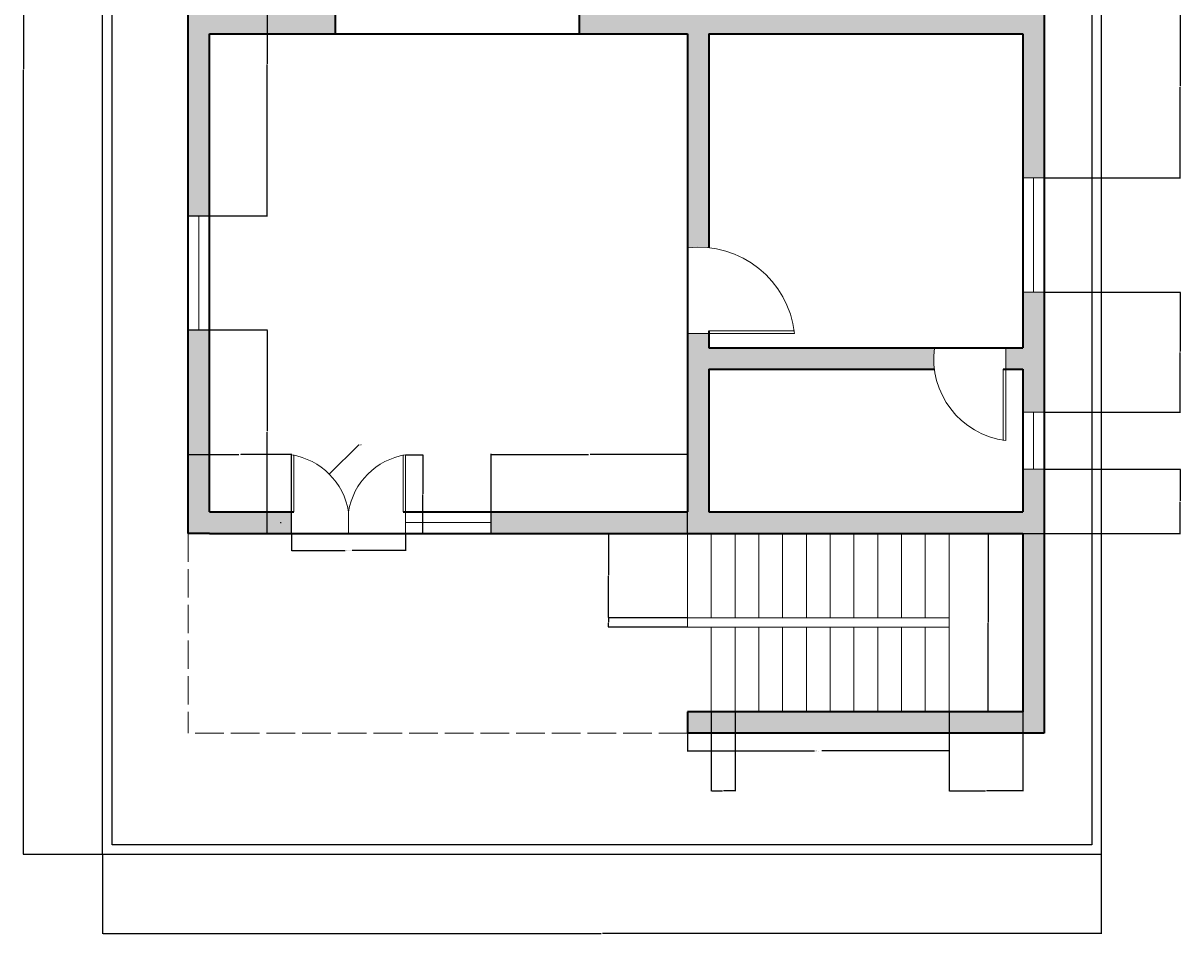
# Model space of a CAD drawing. Units: inches. Extents: x 4948 to 20975, y 6797 to 20508.
# Tile 3 of 5: x 10299 to 10786, y 19781 to 20164. Entities that reach past the tile are written whole.
import ezdxf

# ---------------------------------------------------------------- set-up
doc = ezdxf.new("R2010")
doc.units = ezdxf.units.IN
doc.linetypes.add('ACAD_ISO02W100', pattern=[15, 12, -3])
for name, color, linetype, lineweight in [('A-ANNO-DIMS', 2, 'Continuous', 18), ('A-DOOR', 3, 'Continuous', 18), ('A-FLOR-OVHD', 8, 'ACAD_ISO02W100', 18), ('A-FLOR-STRS', 7, 'Continuous', 18), ('A-GLAZ', 4, 'Continuous', 18), ('A-WALL', 7, 'Continuous', 35), ('C-PROP', 7, 'Continuous', 25)]:
    doc.layers.add(name, color=color, linetype=linetype, lineweight=lineweight)
doc.layers.add('A-WALL-PATT', color=18, linetype='Continuous', lineweight=13, true_color=0x000000)
doc.styles.get("Standard").update_dxf_attribs({"font": 'times.ttf'})
doc.dimstyles.get("Standard").update_dxf_attribs({"dimtxt": 0.18, "dimasz": 0.18, "dimexe": 0.18, "dimexo": 0.0625, "dimgap": 0.09, "dimtad": 0, "dimtih": 1, "dimtoh": 1, "dimdec": 4, "dimzin": 0, "dimdsep": 46, "dimtxsty": 'Standard', "dimcen": 0.09, "dimadec": 0, "dimazin": 0, "dimtfac": 1, "dimtdec": 4, "dimtofl": 0, "dimtmove": 0, "dimatfit": 3, "dimfxl": 1, "dimtolj": 1, "dimtzin": 0, "dimarcsym": 0})

# ---------------------------------------------------------------- blocks, each defined once
blk = doc.blocks.new('DOOR-SINGLE-36IN')
for p, q in [((9, 1), (45, 1)), ((0, 0), (9, 0)), ((9, 0), (45, 0))]:
    blk.add_line(p, q)
blk.add_arc((4.5, -4.5), 40.75, 6.3402, 96.3402)
blk = doc.blocks.new('DOOR-SINGLE-30IN')
for p, q in [((0, 0), (9, 0)), ((9, 1), (39, 1)), ((9, 0), (39, 0))]:
    blk.add_line(p, q)
blk.add_arc((4.5, -4.5), 34.79, 7.4314, 97.4314)
blk = doc.blocks.new('DOOR-DOUBLE-48IN')
for p, q in [((0, 9), (0, 33)), ((1, 9), (1, 33)), ((47, 9), (47, 33)), ((48, 9), (48, 33)), ((0, 9), (0, 0)), ((24, 9), (24, 0)), ((48, 9), (48, 0))]:
    blk.add_line(p, q)
for centre, start, end in [((-4.5, 4.5), 8.9726, 81.0274), ((52.5, 4.5), 98.9726, 171.0274)]:
    blk.add_arc(centre, 28.85, start, end)
blk = doc.blocks.new('WIN-48IN')
for p, q in [((0, 0), (0, 9)), ((48, 0), (48, 9)), ((0, 4.5), (48, 4.5))]:
    blk.add_line(p, q)
blk = doc.blocks.new('WIN-24IN')
for p, q in [((0, 24), (9, 24)), ((4.5, 0), (4.5, 24)), ((0, 0), (9, 0))]:
    blk.add_line(p, q)
blk = doc.blocks.new('WIN-SIDELIGHT-36IN')
for p, q in [((36, 9), (36, 0)), ((0, 4.5), (36, 4.5))]:
    blk.add_line(p, q)
blk = doc.blocks.new('STAIR-RETURN-110IN')
for p, q in [((0, 75), (0, 35.5)), ((10, 75), (10, 39.5)), ((20, 75), (20, 39.5)), ((30, 75), (30, 39.5)), ((40, 75), (40, 39.5)), ((50, 75), (50, 39.5)), ((60, 75), (60, 39.5)), ((70, 75), (70, 39.5)), ((80, 75), (80, 39.5)), ((90, 75), (90, 39.5)), ((100, 75), (100, 39.5)), ((110, 75), (110, 0)), ((110, 39.5), (0, 39.5)), ((110, 35.5), (0, 35.5)), ((10, 35.5), (10, 0)), ((20, 35.5), (20, 0)), ((30, 35.5), (30, 0)), ((40, 35.5), (40, 0)), ((50, 35.5), (50, 0)), ((60, 35.5), (60, 0)), ((70, 35.5), (70, 0)), ((80, 35.5), (80, 0)), ((90, 35.5), (90, 0)), ((100, 35.5), (100, 0))]:
    blk.add_line(p, q)
blk = doc.blocks.new('*D19')
at = {"layer": 'A-ANNO-DIMS', "color": 0, "lineweight": -2, "transparency": 16777216}
for p, q in [((10412.09, 19949.62), (10412.09, 19942.3)), ((10460.09, 19949.62), (10460.09, 19942.3)), ((10412.27, 19942.48), (10434.6, 19942.48)), ((10459.91, 19942.48), (10437.58, 19942.48))]:
    blk.add_line(p, q, dxfattribs=at)
at = {"layer": 'A-ANNO-DIMS', "color": 0, "transparency": 16777216}
for points in [[(10412.27, 19942.51), (10412.27, 19942.45), (10412.09, 19942.48)], [(10459.91, 19942.51), (10459.91, 19942.45), (10460.09, 19942.48)]]:
    blk.add_solid(points, dxfattribs=at)
at = {"layer": 'Defpoints', "color": 0, "transparency": 16777216}
for p in [(10412.09, 19949.68), (10460.09, 19949.68), (10460.09, 19942.48)]:
    blk.add_point(p, dxfattribs=at)
at = {"layer": 'A-ANNO-DIMS', "color": 0, "transparency": 16777216, "insert": (10436.09, 19942.48), "char_height": 0.18, "attachment_point": 5}
blk.add_mtext('\\A1;ENTRY DOORS 48 TYP.', dxfattribs=at)
blk = doc.blocks.new('*D20')
at = {"layer": 'A-ANNO-DIMS', "color": 0, "lineweight": -2, "transparency": 16777216}
for p, q in [((10460.15, 19982.68), (10467.47, 19982.68)), ((10467.29, 19982.5), (10467.29, 19966.36)), ((10467.29, 19949.86), (10467.29, 19966)), ((10460.15, 19949.68), (10467.47, 19949.68))]:
    blk.add_line(p, q, dxfattribs=at)
at = {"layer": 'A-ANNO-DIMS', "color": 0, "transparency": 16777216}
for points in [[(10467.26, 19982.5), (10467.32, 19982.5), (10467.29, 19982.68)], [(10467.26, 19949.86), (10467.32, 19949.86), (10467.29, 19949.68)]]:
    blk.add_solid(points, dxfattribs=at)
at = {"layer": 'Defpoints', "color": 0, "transparency": 16777216}
for p in [(10460.09, 19982.68), (10467.29, 19982.68), (10460.09, 19949.68)]:
    blk.add_point(p, dxfattribs=at)
at = {"layer": 'A-ANNO-DIMS', "color": 0, "transparency": 16777216, "insert": (10467.29, 19966.18), "char_height": 0.18, "attachment_point": 5}
blk.add_mtext('\\A1;33 TYP.', dxfattribs=at)
blk = doc.blocks.new('*D23')
at = {"layer": 'A-ANNO-DIMS', "color": 0, "lineweight": -2, "transparency": 16777216}
for p, q in [((10578.63, 19874.62), (10578.63, 19858)), ((10688.63, 19874.62), (10688.63, 19858)), ((10578.81, 19858.18), (10632.05, 19858.18)), ((10688.45, 19858.18), (10635.2, 19858.18))]:
    blk.add_line(p, q, dxfattribs=at)
at = {"layer": 'A-ANNO-DIMS', "color": 0, "transparency": 16777216}
for points in [[(10578.81, 19858.21), (10578.81, 19858.15), (10578.63, 19858.18)], [(10688.45, 19858.21), (10688.45, 19858.15), (10688.63, 19858.18)]]:
    blk.add_solid(points, dxfattribs=at)
at = {"layer": 'Defpoints', "color": 0, "transparency": 16777216}
for p in [(10578.63, 19874.68), (10688.63, 19874.68), (10688.63, 19858.18)]:
    blk.add_point(p, dxfattribs=at)
at = {"layer": 'A-ANNO-DIMS', "color": 0, "transparency": 16777216, "insert": (10633.63, 19858.18), "char_height": 0.18, "attachment_point": 5}
blk.add_mtext('\\A1;RETURN STAIR 110 TYP.', dxfattribs=at)
blk = doc.blocks.new('*D24')
at = {"layer": 'A-ANNO-DIMS', "color": 0, "lineweight": -2, "transparency": 16777216}
for p, q in [((10688.69, 19949.68), (10705.31, 19949.68)), ((10705.13, 19949.5), (10705.13, 19912.36)), ((10705.13, 19874.86), (10705.13, 19912)), ((10688.69, 19874.68), (10705.31, 19874.68))]:
    blk.add_line(p, q, dxfattribs=at)
at = {"layer": 'A-ANNO-DIMS', "color": 0, "transparency": 16777216}
for points in [[(10705.1, 19949.5), (10705.16, 19949.5), (10705.13, 19949.68)], [(10705.1, 19874.86), (10705.16, 19874.86), (10705.13, 19874.68)]]:
    blk.add_solid(points, dxfattribs=at)
at = {"layer": 'Defpoints', "color": 0, "transparency": 16777216}
for p in [(10688.63, 19949.68), (10705.13, 19949.68), (10688.63, 19874.68)]:
    blk.add_point(p, dxfattribs=at)
at = {"layer": 'A-ANNO-DIMS', "color": 0, "transparency": 16777216, "insert": (10705.13, 19912.18), "char_height": 0.18, "attachment_point": 5}
blk.add_mtext('\\A1;75 TYP.', dxfattribs=at)
blk = doc.blocks.new('*D53')
at = {"layer": 'A-ANNO-DIMS', "color": 0, "lineweight": -2, "transparency": 16777216}
for p, q in [((10332.63, 19814.62), (10332.63, 19781.3)), ((10752.63, 19814.62), (10752.63, 19781.3)), ((10332.81, 19781.48), (10542.34, 19781.48)), ((10752.45, 19781.48), (10542.91, 19781.48))]:
    blk.add_line(p, q, dxfattribs=at)
at = {"layer": 'A-ANNO-DIMS', "color": 0, "transparency": 16777216}
for points in [[(10332.81, 19781.51), (10332.81, 19781.45), (10332.63, 19781.48)], [(10752.45, 19781.51), (10752.45, 19781.45), (10752.63, 19781.48)]]:
    blk.add_solid(points, dxfattribs=at)
at = {"layer": 'Defpoints', "color": 0, "transparency": 16777216}
for p in [(10332.63, 19814.68), (10752.63, 19814.68), (10752.63, 19781.48)]:
    blk.add_point(p, dxfattribs=at)
at = {"layer": 'A-ANNO-DIMS', "color": 0, "transparency": 16777216, "insert": (10542.63, 19781.48), "char_height": 0.18, "attachment_point": 5}
blk.add_mtext('\\A1;420', dxfattribs=at)
blk = doc.blocks.new('*D54')
at = {"layer": 'A-ANNO-DIMS', "color": 0, "lineweight": -2, "transparency": 16777216}
for p, q in [((10332.56, 20474.68), (10299.25, 20474.68)), ((10299.43, 20474.5), (10299.43, 20144.86)), ((10299.43, 19814.86), (10299.43, 20144.5)), ((10332.56, 19814.68), (10299.25, 19814.68))]:
    blk.add_line(p, q, dxfattribs=at)
at = {"layer": 'A-ANNO-DIMS', "color": 0, "transparency": 16777216}
for points in [[(10299.4, 20474.5), (10299.46, 20474.5), (10299.43, 20474.68)], [(10299.4, 19814.86), (10299.46, 19814.86), (10299.43, 19814.68)]]:
    blk.add_solid(points, dxfattribs=at)
at = {"layer": 'Defpoints', "color": 0, "transparency": 16777216}
for p in [(10299.43, 20474.68), (10332.63, 20474.68), (10332.63, 19814.68)]:
    blk.add_point(p, dxfattribs=at)
at = {"layer": 'A-ANNO-DIMS', "color": 0, "transparency": 16777216, "insert": (10299.43, 20144.68), "char_height": 0.18, "attachment_point": 5}
blk.add_mtext('\\A1;660', dxfattribs=at)
blk = doc.blocks.new('*D58')
at = {"layer": 'A-ANNO-DIMS', "color": 0, "lineweight": -2, "transparency": 16777216}
for p, q in [((10368.63, 19949.74), (10368.63, 19983.06)), ((10368.81, 19982.88), (10389.98, 19982.88)), ((10411.91, 19982.88), (10390.74, 19982.88)), ((10412.09, 19949.74), (10412.09, 19983.06))]:
    blk.add_line(p, q, dxfattribs=at)
at = {"layer": 'A-ANNO-DIMS', "color": 0, "transparency": 16777216}
for points in [[(10368.81, 19982.91), (10368.81, 19982.85), (10368.63, 19982.88)], [(10411.91, 19982.91), (10411.91, 19982.85), (10412.09, 19982.88)]]:
    blk.add_solid(points, dxfattribs=at)
at = {"layer": 'Defpoints', "color": 0, "transparency": 16777216}
for p in [(10412.09, 19982.88), (10368.63, 19949.68), (10412.09, 19949.68)]:
    blk.add_point(p, dxfattribs=at)
at = {"layer": 'A-ANNO-DIMS', "color": 0, "transparency": 16777216, "insert": (10390.36, 19982.88), "char_height": 0.18, "attachment_point": 5}
blk.add_mtext('\\A1;43.46', dxfattribs=at)
blk = doc.blocks.new('*D59')
at = {"layer": 'A-ANNO-DIMS', "color": 0, "lineweight": -2, "transparency": 16777216}
for p, q in [((10496.09, 19949.74), (10496.09, 19983.06)), ((10496.27, 19982.88), (10536.98, 19982.88)), ((10578.45, 19982.88), (10537.73, 19982.88)), ((10578.63, 19949.74), (10578.63, 19983.06))]:
    blk.add_line(p, q, dxfattribs=at)
at = {"layer": 'A-ANNO-DIMS', "color": 0, "transparency": 16777216}
for points in [[(10496.27, 19982.91), (10496.27, 19982.85), (10496.09, 19982.88)], [(10578.45, 19982.91), (10578.45, 19982.85), (10578.63, 19982.88)]]:
    blk.add_solid(points, dxfattribs=at)
at = {"layer": 'Defpoints', "color": 0, "transparency": 16777216}
for p in [(10578.63, 19982.88), (10496.09, 19949.68), (10578.63, 19949.68)]:
    blk.add_point(p, dxfattribs=at)
at = {"layer": 'A-ANNO-DIMS', "color": 0, "transparency": 16777216, "insert": (10537.36, 19982.88), "char_height": 0.18, "attachment_point": 5}
blk.add_mtext('\\A1;82.54', dxfattribs=at)
blk = doc.blocks.new('*D62')
at = {"layer": 'A-ANNO-DIMS', "color": 0, "lineweight": -2, "transparency": 16777216}
for p, q in [((10368.69, 20210.68), (10402.01, 20210.68)), ((10401.83, 20210.5), (10401.83, 20147.11)), ((10401.83, 20083.36), (10401.83, 20146.75)), ((10368.69, 20083.18), (10402.01, 20083.18))]:
    blk.add_line(p, q, dxfattribs=at)
at = {"layer": 'A-ANNO-DIMS', "color": 0, "transparency": 16777216}
for points in [[(10401.8, 20210.5), (10401.86, 20210.5), (10401.83, 20210.68)], [(10401.8, 20083.36), (10401.86, 20083.36), (10401.83, 20083.18)]]:
    blk.add_solid(points, dxfattribs=at)
at = {"layer": 'Defpoints', "color": 0, "transparency": 16777216}
for p in [(10368.63, 20210.68), (10368.63, 20083.18), (10401.83, 20083.18)]:
    blk.add_point(p, dxfattribs=at)
at = {"layer": 'A-ANNO-DIMS', "color": 0, "transparency": 16777216, "insert": (10401.83, 20146.93), "char_height": 0.18, "attachment_point": 5}
blk.add_mtext('\\A1;127.5', dxfattribs=at)
blk = doc.blocks.new('*D63')
at = {"layer": 'A-ANNO-DIMS', "color": 0, "lineweight": -2, "transparency": 16777216}
for p, q in [((10368.69, 20035.18), (10402.01, 20035.18)), ((10401.83, 20035), (10401.83, 19992.61)), ((10401.83, 19949.86), (10401.83, 19992.25)), ((10368.69, 19949.68), (10402.01, 19949.68))]:
    blk.add_line(p, q, dxfattribs=at)
at = {"layer": 'A-ANNO-DIMS', "color": 0, "transparency": 16777216}
for points in [[(10401.8, 20035), (10401.86, 20035), (10401.83, 20035.18)], [(10401.8, 19949.86), (10401.86, 19949.86), (10401.83, 19949.68)]]:
    blk.add_solid(points, dxfattribs=at)
at = {"layer": 'Defpoints', "color": 0, "transparency": 16777216}
for p in [(10368.63, 20035.18), (10368.63, 19949.68), (10401.83, 19949.68)]:
    blk.add_point(p, dxfattribs=at)
at = {"layer": 'A-ANNO-DIMS', "color": 0, "transparency": 16777216, "insert": (10401.83, 19992.43), "char_height": 0.18, "attachment_point": 5}
blk.add_mtext('\\A1;85.5', dxfattribs=at)
blk = doc.blocks.new('*D64')
at = {"layer": 'A-ANNO-DIMS', "color": 0, "lineweight": -2, "transparency": 16777216}
for p, q in [((10728.69, 19976.68), (10786.01, 19976.68)), ((10785.83, 19976.5), (10785.83, 19963.36)), ((10785.83, 19949.86), (10785.83, 19963)), ((10719.69, 19949.68), (10786.01, 19949.68))]:
    blk.add_line(p, q, dxfattribs=at)
at = {"layer": 'A-ANNO-DIMS', "color": 0, "transparency": 16777216}
for points in [[(10785.8, 19976.5), (10785.86, 19976.5), (10785.83, 19976.68)], [(10785.8, 19949.86), (10785.86, 19949.86), (10785.83, 19949.68)]]:
    blk.add_solid(points, dxfattribs=at)
at = {"layer": 'Defpoints', "color": 0, "transparency": 16777216}
for p in [(10728.63, 19976.68), (10719.63, 19949.68), (10785.83, 19949.68)]:
    blk.add_point(p, dxfattribs=at)
at = {"layer": 'A-ANNO-DIMS', "color": 0, "transparency": 16777216, "insert": (10785.83, 19963.18), "char_height": 0.18, "attachment_point": 5}
blk.add_mtext('\\A1;27', dxfattribs=at)
blk = doc.blocks.new('*D65')
at = {"layer": 'A-ANNO-DIMS', "color": 0, "lineweight": -2, "transparency": 16777216}
for p, q in [((10728.69, 20051.13), (10786.01, 20051.13)), ((10785.83, 20050.95), (10785.83, 20026.09)), ((10785.83, 20000.86), (10785.83, 20025.72)), ((10728.69, 20000.68), (10786.01, 20000.68))]:
    blk.add_line(p, q, dxfattribs=at)
at = {"layer": 'A-ANNO-DIMS', "color": 0, "transparency": 16777216}
for points in [[(10785.8, 20050.95), (10785.86, 20050.95), (10785.83, 20051.13)], [(10785.8, 20000.86), (10785.86, 20000.86), (10785.83, 20000.68)]]:
    blk.add_solid(points, dxfattribs=at)
at = {"layer": 'Defpoints', "color": 0, "transparency": 16777216}
for p in [(10728.63, 20051.13), (10785.83, 20051.13), (10728.63, 20000.68)]:
    blk.add_point(p, dxfattribs=at)
at = {"layer": 'A-ANNO-DIMS', "color": 0, "transparency": 16777216, "insert": (10785.83, 20025.91), "char_height": 0.18, "attachment_point": 5}
blk.add_mtext('\\A1;50.45', dxfattribs=at)
blk = doc.blocks.new('*D66')
at = {"layer": 'A-ANNO-DIMS', "color": 0, "lineweight": -2, "transparency": 16777216}
for p, q in [((10728.69, 20175.78), (10786.01, 20175.78)), ((10785.83, 20175.6), (10785.83, 20137.64)), ((10785.83, 20099.31), (10785.83, 20137.27)), ((10728.69, 20099.13), (10786.01, 20099.13))]:
    blk.add_line(p, q, dxfattribs=at)
at = {"layer": 'A-ANNO-DIMS', "color": 0, "transparency": 16777216}
for points in [[(10785.8, 20175.6), (10785.86, 20175.6), (10785.83, 20175.78)], [(10785.8, 20099.31), (10785.86, 20099.31), (10785.83, 20099.13)]]:
    blk.add_solid(points, dxfattribs=at)
at = {"layer": 'Defpoints', "color": 0, "transparency": 16777216}
for p in [(10728.63, 20175.78), (10785.83, 20175.78), (10728.63, 20099.13)]:
    blk.add_point(p, dxfattribs=at)
at = {"layer": 'A-ANNO-DIMS', "color": 0, "transparency": 16777216, "insert": (10785.83, 20137.46), "char_height": 0.18, "attachment_point": 5}
blk.add_mtext('\\A1;76.65', dxfattribs=at)
blk = doc.blocks.new('*D69')
at = {"layer": 'A-ANNO-DIMS', "color": 0, "lineweight": -2, "transparency": 16777216}
for p, q in [((10578.56, 19949.68), (10545.25, 19949.68)), ((10545.43, 19949.5), (10545.43, 19932.11)), ((10545.43, 19914.36), (10545.43, 19931.75)), ((10578.56, 19914.18), (10545.25, 19914.18))]:
    blk.add_line(p, q, dxfattribs=at)
at = {"layer": 'A-ANNO-DIMS', "color": 0, "transparency": 16777216}
for points in [[(10545.4, 19949.5), (10545.46, 19949.5), (10545.43, 19949.68)], [(10545.4, 19914.36), (10545.46, 19914.36), (10545.43, 19914.18)]]:
    blk.add_solid(points, dxfattribs=at)
at = {"layer": 'Defpoints', "color": 0, "transparency": 16777216}
for p in [(10545.43, 19949.68), (10578.63, 19949.68), (10578.63, 19914.18)]:
    blk.add_point(p, dxfattribs=at)
at = {"layer": 'A-ANNO-DIMS', "color": 0, "transparency": 16777216, "insert": (10545.43, 19931.93), "char_height": 0.18, "attachment_point": 5}
blk.add_mtext('\\A1;35.5', dxfattribs=at)
blk = doc.blocks.new('*D70')
at = {"layer": 'A-ANNO-DIMS', "color": 0, "lineweight": -2, "transparency": 16777216}
for p, q in [((10578.564704, 19914.180248), (10545.247204, 19914.180248)), ((10578.564704, 19910.180248), (10545.247204, 19910.180248)), ((10545.427204, 19914.000248), (10545.427204, 19912.360248)), ((10545.427204, 19910.360248), (10545.427204, 19912.000248))]:
    blk.add_line(p, q, dxfattribs=at)
at = {"layer": 'A-ANNO-DIMS', "color": 0, "transparency": 16777216}
for points in [[(10545.397204, 19914.000248), (10545.457204, 19914.000248), (10545.427204, 19914.180248)], [(10545.397204, 19910.360248), (10545.457204, 19910.360248), (10545.427204, 19910.180248)]]:
    blk.add_solid(points, dxfattribs=at)
at = {"layer": 'Defpoints', "color": 0, "transparency": 16777216}
for p in [(10545.427204, 19914.180248), (10578.627204, 19914.180248), (10578.627204, 19910.180248)]:
    blk.add_point(p, dxfattribs=at)
at = {"layer": 'A-ANNO-DIMS', "color": 0, "transparency": 16777216, "insert": (10545.427204, 19912.180248), "char_height": 0.18, "attachment_point": 5}
blk.add_mtext('\\A1;4', dxfattribs=at)
blk = doc.blocks.new('*D71')
at = {"layer": 'A-ANNO-DIMS', "color": 0, "lineweight": -2, "transparency": 16777216}
for p, q in [((10588.63, 19874.62), (10588.63, 19841.3)), ((10598.63, 19874.62), (10598.63, 19841.3)), ((10588.81, 19841.48), (10593.42, 19841.48)), ((10598.45, 19841.48), (10593.83, 19841.48))]:
    blk.add_line(p, q, dxfattribs=at)
at = {"layer": 'A-ANNO-DIMS', "color": 0, "transparency": 16777216}
for points in [[(10588.81, 19841.51), (10588.81, 19841.45), (10588.63, 19841.48)], [(10598.45, 19841.51), (10598.45, 19841.45), (10598.63, 19841.48)]]:
    blk.add_solid(points, dxfattribs=at)
at = {"layer": 'Defpoints', "color": 0, "transparency": 16777216}
for p in [(10588.63, 19874.68), (10598.63, 19874.68), (10588.63, 19841.48)]:
    blk.add_point(p, dxfattribs=at)
at = {"layer": 'A-ANNO-DIMS', "color": 0, "transparency": 16777216, "insert": (10593.63, 19841.48), "char_height": 0.18, "attachment_point": 5}
blk.add_mtext('\\A1;10', dxfattribs=at)
blk = doc.blocks.new('*D72')
at = {"layer": 'A-ANNO-DIMS', "color": 0, "lineweight": -2, "transparency": 16777216}
for p, q in [((10688.63, 19874.62), (10688.63, 19841.3)), ((10719.63, 19874.62), (10719.63, 19841.3)), ((10688.81, 19841.48), (10703.93, 19841.48)), ((10719.45, 19841.48), (10704.33, 19841.48))]:
    blk.add_line(p, q, dxfattribs=at)
at = {"layer": 'A-ANNO-DIMS', "color": 0, "transparency": 16777216}
for points in [[(10688.81, 19841.51), (10688.81, 19841.45), (10688.63, 19841.48)], [(10719.45, 19841.51), (10719.45, 19841.45), (10719.63, 19841.48)]]:
    blk.add_solid(points, dxfattribs=at)
at = {"layer": 'Defpoints', "color": 0, "transparency": 16777216}
for p in [(10688.63, 19874.68), (10719.63, 19874.68), (10688.63, 19841.48)]:
    blk.add_point(p, dxfattribs=at)
at = {"layer": 'A-ANNO-DIMS', "color": 0, "transparency": 16777216, "insert": (10704.13, 19841.48), "char_height": 0.18, "attachment_point": 5}
blk.add_mtext('\\A1;31', dxfattribs=at)
blk = doc.blocks.new('*D95')
at = {"layer": 'A-ANNO-DIMS', "color": 0, "lineweight": -2, "transparency": 16777216}
for p, q in [((10440.23, 19986.82), (10428.12, 19974.71)), ((10440.41, 19986.82), (10440.23, 19986.82)), ((10407.5, 19954.18), (10407.68, 19954.18)), ((10407.59, 19954.09), (10407.59, 19954.27))]:
    blk.add_line(p, q, dxfattribs=at)
at = {"layer": 'A-ANNO-DIMS', "color": 0, "transparency": 16777216}
blk.add_solid([(10428.1, 19974.73), (10428.14, 19974.69), (10427.99, 19974.58)], dxfattribs=at)
at = {"layer": 'Defpoints', "color": 0, "transparency": 16777216}
for p in [(10427.99, 19974.58), (10407.59, 19954.18)]:
    blk.add_point(p, dxfattribs=at)
at = {"layer": 'A-ANNO-DIMS', "color": 0, "transparency": 16777216, "insert": (10441.14, 19986.82), "char_height": 0.18, "attachment_point": 5}
blk.add_mtext('\\A1;2X R28.853', dxfattribs=at)

msp = doc.modelspace()

# ---------------------------------------------------------------- hatches: boundary and pattern name
at = {"layer": 'A-WALL-PATT'}
h = msp.add_hatch(color=256, dxfattribs=at)
h.dxf.hatch_style = 1
h.paths.add_polyline_path([(10447.2486, 20450.6802), (10368.6272, 20450.6802), (10368.6272, 20386.7714), (10377.6272, 20386.7714), (10377.6272, 20441.6802), (10447.2486, 20441.6802)])
h.paths.add_polyline_path([(10598.2871, 20450.6802), (10495.2486, 20450.6802), (10495.2486, 20441.6802), (10509.6272, 20441.6802), (10509.6272, 20358.7457, -0.06494234), (10518.6272, 20358.7457), (10518.6272, 20441.6802), (10578.6272, 20441.6802), (10578.6272, 20321.6802), (10518.6272, 20321.6802), (10518.6272, 20328.7457), (10509.6272, 20328.7457), (10509.6272, 20321.6802), (10498.0955, 20321.6802), (10498.0955, 20312.6802), (10578.6272, 20312.6802), (10578.6272, 20280.7888, -0.05538514), (10587.6272, 20280.7888), (10587.6272, 20312.6802), (10587.6272, 20441.6802), (10598.2871, 20441.6802)])
h.paths.add_polyline_path([(10728.6272, 20450.6802), (10646.2871, 20450.6802), (10646.2871, 20441.6802), (10719.6272, 20441.6802), (10719.6272, 20302.385), (10728.6272, 20302.385)])
h.paths.add_polyline_path([(10377.6272, 20312.6802), (10462.0955, 20312.6802), (10462.0955, 20321.6802), (10377.6272, 20321.6802), (10377.6272, 20338.7714), (10368.6272, 20338.7714), (10368.6272, 20270.6802), (10377.6272, 20270.6802)])
h.paths.add_polyline_path([(10728.6272, 20175.7784), (10719.6272, 20175.7784), (10719.6272, 20168.6802), (10587.6272, 20168.6802), (10587.6272, 20228.6802), (10680.8649, 20228.6802, -0.06494234), (10680.8649, 20237.6802), (10587.6272, 20237.6802), (10587.6272, 20244.7888), (10578.6272, 20244.7888), (10578.6272, 20228.6802), (10578.6272, 20168.6802), (10533.2309, 20168.6802), (10533.2309, 20159.6802), (10578.6272, 20159.6802), (10578.6272, 20069.7581, -0.05538514), (10587.6272, 20069.7581), (10587.6272, 20159.6802), (10719.6272, 20159.6802), (10719.6272, 20099.1317), (10728.6272, 20099.1317)])
h.paths.add_polyline_path([(10728.6272, 20254.385), (10719.6272, 20254.385), (10719.6272, 20237.6802), (10710.8649, 20237.6802), (10710.8649, 20228.6802), (10719.6272, 20228.6802), (10719.6272, 20199.7784), (10728.6272, 20199.7784)])
h.paths.add_polyline_path([(10728.6272, 20051.1317), (10719.6272, 20051.1317), (10719.6272, 20027.6802), (10712.464, 20027.6802), (10712.464, 20018.6802), (10719.6272, 20018.6802), (10719.6272, 20000.6802), (10728.6272, 20000.6802)])
h.paths.add_polyline_path([(10728.6272, 19976.6802), (10719.6272, 19976.6802), (10719.6272, 19958.6802), (10587.6272, 19958.6802), (10587.6272, 20018.6802), (10682.464, 20018.6802, -0.06494234), (10682.464, 20027.6802), (10587.6272, 20027.6802), (10587.6272, 20033.7581), (10578.6272, 20033.7581), (10578.6272, 19958.6802), (10496.0899, 19958.6802), (10496.0899, 19949.6802), (10578.6272, 19949.6802), (10587.6272, 19949.6802), (10719.6272, 19949.6802), (10719.6272, 19874.6802), (10578.6272, 19874.6802), (10578.6272, 19865.6802), (10728.6272, 19865.6802)])
h.paths.add_polyline_path([(10412.0899, 19958.6802), (10377.6272, 19958.6802), (10377.6272, 20035.1802), (10368.6272, 20035.1802), (10368.6272, 19949.6802), (10377.6272, 19949.6802), (10412.0899, 19949.6802)])
h.paths.add_polyline_path([(10377.6272, 20159.6802), (10430.5935, 20159.6802), (10430.5935, 20168.6802), (10377.6272, 20168.6802), (10377.6272, 20210.6802), (10368.6272, 20210.6802), (10368.6272, 20083.1802), (10377.6272, 20083.1802)])

# ---------------------------------------------------------------- linework, layer by layer
at = {"layer": 'A-FLOR-OVHD'}
for p in [(10368.6272, 19949.6802), (10578.6272, 19865.6802)]:
    msp.add_line(p, (10368.6272, 19865.6802), dxfattribs=at)
at = {"layer": 'A-WALL'}
for p, q in [((10368.6272, 19949.6802), (10368.6272, 20450.6802)), ((10728.6272, 20450.6802), (10728.6272, 19865.6802)), ((10430.5935, 20159.6802), (10430.5935, 20168.6802)), ((10533.2309, 20159.6802), (10533.2309, 20168.6802)), ((10377.6272, 20159.6802), (10430.5935, 20159.6802)), ((10377.6272, 19958.6802), (10377.6272, 20159.6802)), ((10430.5935, 20159.6802), (10533.2309, 20159.6802)), ((10533.2309, 20159.6802), (10578.6272, 20159.6802)), ((10578.6272, 20159.6802), (10578.6272, 19958.6802)), ((10587.6272, 20159.6802), (10587.6272, 20069.7581)), ((10587.6272, 20159.6802), (10719.6272, 20159.6802)), ((10719.6272, 20159.6802), (10719.6272, 20027.6802)), ((10587.6272, 20034.7581), (10587.6272, 20027.6802)), ((10587.6272, 20027.6802), (10719.6272, 20027.6802)), ((10587.6272, 20018.6802), (10587.6272, 19958.6802)), ((10587.6272, 20018.6802), (10682.464, 20018.6802)), ((10711.464, 20018.6802), (10719.6272, 20018.6802)), ((10719.6272, 20018.6802), (10719.6272, 19958.6802)), ((10377.6272, 19958.6802), (10413.0899, 19958.6802)), ((10459.0899, 19958.6802), (10578.6272, 19958.6802)), ((10587.6272, 19958.6802), (10719.6272, 19958.6802)), ((10377.6272, 19949.6802), (10368.6272, 19949.6802)), ((10377.6272, 19949.6802), (10578.6272, 19949.6802)), ((10578.6272, 19949.6802), (10587.6272, 19949.6802)), ((10587.6272, 19949.6802), (10719.6272, 19949.6802)), ((10719.6272, 19949.6802), (10719.6272, 19874.6802)), ((10719.6272, 19874.6802), (10578.6272, 19874.6802)), ((10578.6272, 19874.6802), (10578.6272, 19865.6802)), ((10728.6272, 19865.6802), (10578.6272, 19865.6802))]:
    msp.add_line(p, q, dxfattribs=at)
at = {"layer": 'C-PROP'}
for p, q in [((10332.6272, 19814.6802), (10332.6272, 20474.6802)), ((10752.6272, 20474.6802), (10752.6272, 19814.6802)), ((10336.6272, 19818.6802), (10336.6272, 20470.6802)), ((10748.6272, 20470.6802), (10748.6272, 19818.6802)), ((10748.6272, 19818.6802), (10336.6272, 19818.6802)), ((10752.6272, 19814.6802), (10332.6272, 19814.6802))]:
    msp.add_line(p, q, dxfattribs=at)

# ---------------------------------------------------------------- block references
at = {"layer": 'A-DOOR'}
for name, p in [('DOOR-SINGLE-36IN', (10578.6273, 20033.7584)), ('DOOR-DOUBLE-48IN', (10412.0903, 19949.6802))]:
    msp.add_blockref(name, p, dxfattribs=at)
at = {"layer": 'A-DOOR', "extrusion": (0, 0, -1), "zscale": -1, "rotation": 270.0000000000293}
msp.add_blockref('DOOR-SINGLE-30IN', (-10712.4645, 20027.6802), dxfattribs=at)
at = {"layer": 'A-FLOR-STRS'}
msp.add_blockref('STAIR-RETURN-110IN', (10578.6273, 19874.6802), dxfattribs=at)
at = {"layer": 'A-GLAZ'}
for name, p, rotation in [('WIN-48IN', (10719.6272, 20099.1321), 269.9999999999971), ('WIN-48IN', (10377.6272, 20035.1799), 89.99999999999031), ('WIN-24IN', (10728.6271, 20000.6804), 180)]:
    msp.add_blockref(name, p, dxfattribs=dict(at, rotation=rotation))
msp.add_blockref('WIN-SIDELIGHT-36IN', (10460.0903, 19949.6802), dxfattribs=at)

# ---------------------------------------------------------------- dimensions: what is measured, and where the dimension line sits
at = {"layer": 'A-ANNO-DIMS'}
for base, p1, p2, angle, override, picture, middle in [((10299.4272, 20474.6802), (10332.6272, 19814.6802), (10332.6272, 20474.6802), 90, {"dimdec": 0, "dimlfac": 1, "dimrnd": 0, "dimzin": 0, "dimdsep": 46, "dimlunit": 2}, '*D54', (10299.4272, 20144.6802)), ((10401.8272, 20083.1802), (10368.6272, 20210.6802), (10368.6272, 20083.1802), 270, {"dimdec": 1, "dimlfac": 1, "dimrnd": 0, "dimzin": 0, "dimdsep": 46, "dimlunit": 2}, '*D62', (10401.8272, 20146.9302)), ((10785.8272, 20175.7784), (10728.6272, 20099.1317), (10728.6272, 20175.7784), 90, {"dimdec": 2, "dimlfac": 1, "dimrnd": 0, "dimzin": 0, "dimdsep": 46, "dimlunit": 2}, '*D66', (10785.8272, 20137.4551)), ((10785.8272, 20051.1317), (10728.6272, 20000.6802), (10728.6272, 20051.1317), 90, {"dimdec": 2, "dimlfac": 1, "dimrnd": 0, "dimzin": 0, "dimdsep": 46, "dimlunit": 2}, '*D65', (10785.8272, 20025.906)), ((10401.8272, 19949.6802), (10368.6272, 20035.1802), (10368.6272, 19949.6802), 270, {"dimdec": 1, "dimlfac": 1, "dimrnd": 0, "dimzin": 0, "dimdsep": 46, "dimlunit": 2}, '*D63', (10401.8272, 19992.4302)), ((10412.0899, 19982.8802), (10368.6272, 19949.6802), (10412.0899, 19949.6802), 0, {"dimdec": 2, "dimlfac": 1, "dimrnd": 0, "dimzin": 0, "dimdsep": 46, "dimlunit": 2}, '*D58', (10390.3586, 19982.8802)), ((10578.6272, 19982.8802), (10496.0899, 19949.6802), (10578.6272, 19949.6802), 0, {"dimdec": 2, "dimlfac": 1, "dimrnd": 0, "dimzin": 0, "dimdsep": 46, "dimlunit": 2}, '*D59', (10537.3586, 19982.8802)), ((10785.8272, 19949.6802), (10728.6272, 19976.6802), (10719.6272, 19949.6802), 90, {"dimdec": 0, "dimlfac": 1, "dimrnd": 0, "dimzin": 0, "dimdsep": 46, "dimlunit": 2}, '*D64', (10785.8272, 19963.1802)), ((10545.4272, 19949.6802), (10578.6272, 19914.1802), (10578.6272, 19949.6802), 90, {"dimdec": 1, "dimlfac": 1, "dimrnd": 0, "dimzin": 0, "dimdsep": 46, "dimlunit": 2}, '*D69', (10545.4272, 19931.9302)), ((10545.4272, 19914.1802), (10578.6272, 19910.1802), (10578.6272, 19914.1802), 90, {"dimdec": 0, "dimlfac": 1, "dimrnd": 0, "dimzin": 0, "dimdsep": 46, "dimlunit": 2}, '*D70', (10545.4272, 19912.1802)), ((10588.6272, 19841.4802), (10598.6272, 19874.6802), (10588.6272, 19874.6802), 180, {"dimdec": 0, "dimlfac": 1, "dimrnd": 0, "dimzin": 0, "dimdsep": 46, "dimlunit": 2}, '*D71', (10593.6272, 19841.4802)), ((10688.6272, 19841.4802), (10719.6272, 19874.6802), (10688.6272, 19874.6802), 180, {"dimdec": 0, "dimlfac": 1, "dimrnd": 0, "dimzin": 0, "dimdsep": 46, "dimlunit": 2}, '*D72', (10704.1272, 19841.4802))]:
    dim = msp.add_linear_dim(base=base, p1=p1, p2=p2, angle=angle, dimstyle='Standard', override=override, dxfattribs=at)
    dim.commit()
    dim.dimension.update_dxf_attribs({"geometry": picture, "text_midpoint": middle})
dim = msp.add_radius_dim(center=(10407.5899, 19954.1802), mpoint=(10427.9923, 19974.5823), text='2X <>', dimstyle='Standard', override={"dimdec": 3, "dimlfac": 1, "dimrnd": 0, "dimzin": 0, "dimdsep": 46, "dimlunit": 2}, dxfattribs=at)
dim.commit()
dim.dimension.update_dxf_attribs({"geometry": '*D95', "text_midpoint": (10441.1396, 19986.8235), "dimtype": 164})
for base, p1, p2, picture, middle in [((10467.2899, 19982.6802), (10460.0899, 19949.6802), (10460.0899, 19982.6802), '*D20', (10467.2899, 19966.1802)), ((10705.1272, 19949.6802), (10688.6272, 19874.6802), (10688.6272, 19949.6802), '*D24', (10705.1272, 19912.1802))]:
    dim = msp.add_linear_dim(base=base, p1=p1, p2=p2, angle=90, text='<> TYP.', dimstyle='Standard', override={"dimdec": 0, "dimlfac": 1, "dimrnd": 0, "dimzin": 0, "dimdsep": 46, "dimlunit": 2}, dxfattribs=at)
    dim.commit()
    dim.dimension.update_dxf_attribs({"geometry": picture, "text_midpoint": middle})
for base, p1, p2, text, picture, middle in [((10460.0899, 19942.4802), (10412.0899, 19949.6802), (10460.0899, 19949.6802), 'ENTRY DOORS <> TYP.', '*D19', (10436.0899, 19942.4802)), ((10688.6272, 19858.1802), (10578.6272, 19874.6802), (10688.6272, 19874.6802), 'RETURN STAIR <> TYP.', '*D23', (10633.6272, 19858.1802))]:
    dim = msp.add_linear_dim(base=base, p1=p1, p2=p2, text=text, dimstyle='Standard', override={"dimdec": 0, "dimlfac": 1, "dimrnd": 0, "dimzin": 0, "dimdsep": 46, "dimlunit": 2}, dxfattribs=at)
    dim.commit()
    dim.dimension.update_dxf_attribs({"geometry": picture, "text_midpoint": middle})
dim = msp.add_linear_dim(base=(10752.6272, 19781.4802), p1=(10332.6272, 19814.6802), p2=(10752.6272, 19814.6802), dimstyle='Standard', override={"dimdec": 0, "dimlfac": 1, "dimrnd": 0, "dimzin": 0, "dimdsep": 46, "dimlunit": 2}, dxfattribs=at)
dim.commit()
dim.dimension.update_dxf_attribs({"geometry": '*D53', "text_midpoint": (10542.6272, 19781.4802)})

doc.saveas('drawing.dxf')
